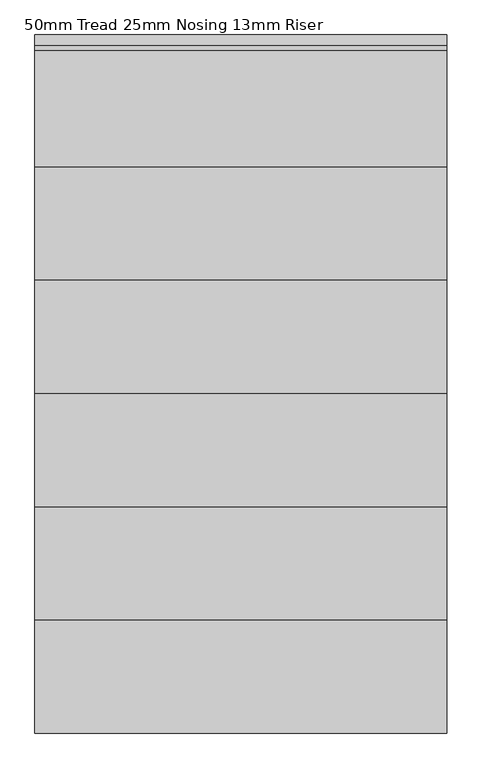
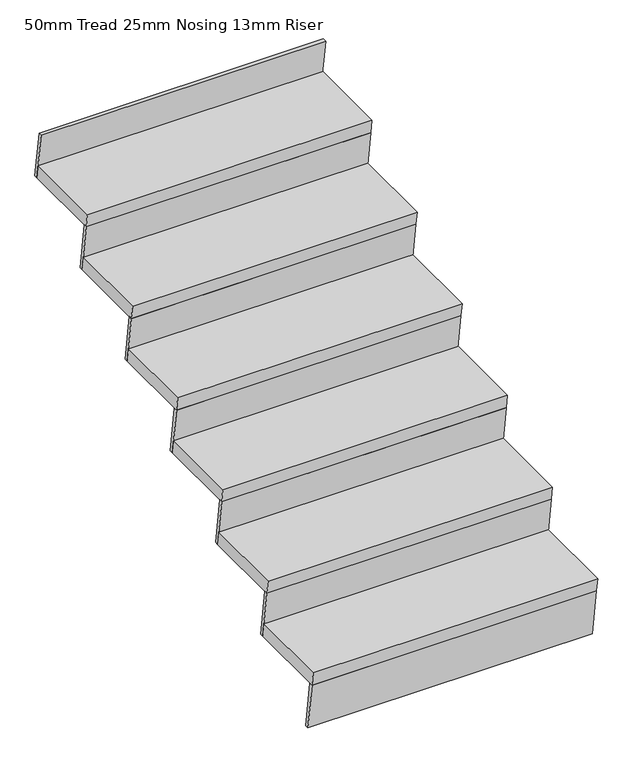
"""IFC4 building model written with IfcOpenShell, lengths in millimetres: stair flight geometry, 50mm Tread 25mm Nosing 13mm Riser."""

from ifc_helpers import new_model, si_unit, frame, origin, place, context, project, spatial, polyline, outline, extrude, source, transform, mapped, element, save


def stair_flight_50mm_tread_25mm_nosing_13mm_riser_0ce5104d(model_context):
    return source(origin(), model_context, "Body", "SweptSolid", [
        extrude(outline(polyline([(4453.248464, 1913.0434783), (4753.248464, 1913.0434783), (4760.435964, 1863.0434783), (4460.435964, 1863.0434783), (4453.248464, 1913.0434783)])), frame((2126.013846, 0.0, 0.0), z_axis=(1.0, 0.0, 0.0), x_axis=(0.0, 1.0, 0.0)), (0.0, 0.0, 1.0), 1000.0257813),
        extrude(outline(polyline([(4460.435964, 1863.0434783), (4473.064454, 1863.0434783), (4498.064454, 1689.1304348), (4485.435964, 1689.1304348), (4460.435964, 1863.0434783)])), frame((2126.013846, 0.0, 0.0), z_axis=(1.0, 0.0, 0.0), x_axis=(0.0, 1.0, 0.0)), (0.0, 0.0, 1.0), 1000.0257813),
        extrude(outline(polyline([(4735.435964, 2036.9565217), (4748.064454, 2036.9565217), (4773.064454, 1863.0434783), (4760.435964, 1863.0434783), (4735.435964, 2036.9565217)])), frame((2126.013846, 0.0, 0.0), z_axis=(1.0, 0.0, 0.0), x_axis=(0.0, 1.0, 0.0)), (0.0, 0.0, 1.0), 1000.0257812),
        extrude(outline(polyline([(4728.248464, 2086.9565217), (5028.248464, 2086.9565217), (5035.435964, 2036.9565217), (4735.435964, 2036.9565217), (4728.248464, 2086.9565217)])), frame((2126.013846, 0.0, 0.0), z_axis=(1.0, 0.0, 0.0), x_axis=(0.0, 1.0, 0.0)), (0.0, 0.0, 1.0), 1000.0257812),
        extrude(outline(polyline([(5010.435964, 2210.8695652), (5023.064454, 2210.8695652), (5048.064454, 2036.9565217), (5035.435964, 2036.9565217), (5010.435964, 2210.8695652)])), frame((2126.013846, 0.0, 0.0), z_axis=(1.0, 0.0, 0.0), x_axis=(0.0, 1.0, 0.0)), (0.0, 0.0, 1.0), 1000.0257812),
        extrude(outline(polyline([(5003.248464, 2260.8695652), (5303.248464, 2260.8695652), (5310.435964, 2210.8695652), (5010.435964, 2210.8695652), (5003.248464, 2260.8695652)])), frame((2126.013846, 0.0, 0.0), z_axis=(1.0, 0.0, 0.0), x_axis=(0.0, 1.0, 0.0)), (0.0, 0.0, 1.0), 1000.0257812),
        extrude(outline(polyline([(5285.435964, 2384.7826087), (5298.064454, 2384.7826087), (5323.064454, 2210.8695652), (5310.435964, 2210.8695652), (5285.435964, 2384.7826087)])), frame((2126.013846, 0.0, 0.0), z_axis=(1.0, 0.0, 0.0), x_axis=(0.0, 1.0, 0.0)), (0.0, 0.0, 1.0), 1000.0257812),
        extrude(outline(polyline([(5278.248464, 2434.7826087), (5578.248464, 2434.7826087), (5585.435964, 2384.7826087), (5285.435964, 2384.7826087), (5278.248464, 2434.7826087)])), frame((2126.013846, 0.0, 0.0), z_axis=(1.0, 0.0, 0.0), x_axis=(0.0, 1.0, 0.0)), (0.0, 0.0, 1.0), 1000.0257812),
        extrude(outline(polyline([(5560.435964, 2558.6956522), (5573.064454, 2558.6956522), (5598.064454, 2384.7826087), (5585.435964, 2384.7826087), (5560.435964, 2558.6956522)])), frame((2126.013846, 0.0, 0.0), z_axis=(1.0, 0.0, 0.0), x_axis=(0.0, 1.0, 0.0)), (0.0, 0.0, 1.0), 1000.0257812),
        extrude(outline(polyline([(5553.248464, 2608.6956522), (5853.248464, 2608.6956522), (5860.435964, 2558.6956522), (5560.435964, 2558.6956522), (5553.248464, 2608.6956522)])), frame((2126.013846, 0.0, 0.0), z_axis=(1.0, 0.0, 0.0), x_axis=(0.0, 1.0, 0.0)), (0.0, 0.0, 1.0), 1000.0257812),
        extrude(outline(polyline([(5835.435964, 2732.6086957), (5848.064454, 2732.6086957), (5873.064454, 2558.6956522), (5860.435964, 2558.6956522), (5835.435964, 2732.6086957)])), frame((2126.013846, 0.0, 0.0), z_axis=(1.0, 0.0, 0.0), x_axis=(0.0, 1.0, 0.0)), (0.0, 0.0, 1.0), 1000.0257813),
        extrude(outline(polyline([(6110.435964, 2906.5217391), (6123.064454, 2906.5217391), (6148.064454, 2732.6086957), (6135.435964, 2732.6086957), (6110.435964, 2906.5217391)])), frame((2126.013846, 0.0, 0.0), z_axis=(1.0, 0.0, 0.0), x_axis=(0.0, 1.0, 0.0)), (0.0, 0.0, 1.0), 1000.0257813),
        extrude(outline(polyline([(5828.248464, 2782.6086957), (6128.248464, 2782.6086957), (6135.435964, 2732.6086957), (5835.435964, 2732.6086957), (5828.248464, 2782.6086957)])), frame((2126.013846, 0.0, 0.0), z_axis=(1.0, 0.0, 0.0), x_axis=(0.0, 1.0, 0.0)), (0.0, 0.0, 1.0), 1000.0257813),
    ])


if __name__ == "__main__":
    model = new_model("IFC4")
    model_context = context("Model", 3, world=origin())
    ifc_project = project(units=[si_unit("LENGTHUNIT", "METRE", prefix="MILLI")], contexts=[model_context])
    site = spatial("IfcSite", under=ifc_project)
    building = spatial("IfcBuilding", under=site)
    placement = place(None, origin())
    stair_flight_50mm_tread_25mm_nosing_13mm_riser_shape = stair_flight_50mm_tread_25mm_nosing_13mm_riser_0ce5104d(model_context)
    element("IfcStairFlight", 1, ObjectType="50mm Tread 25mm Nosing 13mm Riser", at=placement, inside=building, context=model_context, shape_type="MappedRepresentation", body=[
        mapped(stair_flight_50mm_tread_25mm_nosing_13mm_riser_shape, transform((0.0, 0.0, 0.0), x_axis=(1.0, 0.0, 0.0), y_axis=(0.0, 1.0, 0.0), z_axis=(0.0, 0.0, 1.0))),
    ])
    save(model, "model.ifc")
